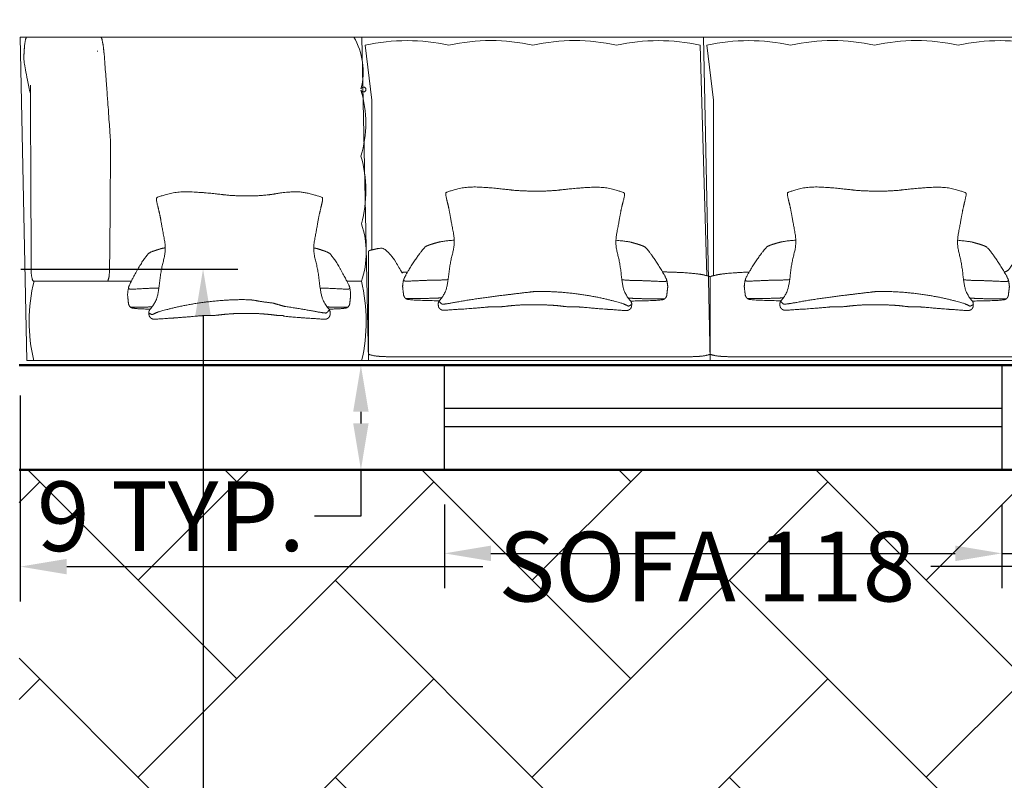
# Model space of a CAD drawing. Units: inches. Extents: x -466983 to 1020, y 324 to 318697.
# Tile 26 of 97: x 814 to 899, y 592 to 658. Entities that reach past the tile are written whole.
import ezdxf

# ---------------------------------------------------------------- set-up
doc = ezdxf.new("R2010")
doc.units = ezdxf.units.IN
doc.header["$MEASUREMENT"] = 0
for name, color, linetype, lineweight in [('A-ANNO-DIMS', 2, 'Continuous', 18), ('A-FLOR-PATT', 252, 'Continuous', 13), ('A-FURN', 8, 'Continuous', 18), ('A-GLAZ', 4, 'Continuous', 25), ('A-WALL', 7, 'Continuous', 50)]:
    doc.layers.add(name, color=color, linetype=linetype, lineweight=lineweight)
doc.styles.get("Standard").update_dxf_attribs({"font": 'arial.ttf'})
doc.dimstyles.get("Standard").update_dxf_attribs({"dimtxt": 6, "dimasz": 4, "dimexe": 3, "dimexo": 3, "dimgap": 0.09, "dimtad": 0, "dimtih": 1, "dimtoh": 1, "dimdec": 1, "dimzin": 0, "dimdsep": 46, "dimlunit": 3, "dimtxsty": 'Standard', "dimcen": 0.09, "dimadec": 0, "dimazin": 0, "dimtfac": 1, "dimtdec": 1, "dimtofl": 0, "dimtmove": 0, "dimatfit": 3, "dimfxl": 1, "dimtolj": 1, "dimtzin": 0, "dimarcsym": 0})

# ---------------------------------------------------------------- blocks, each defined once
blk = doc.blocks.new('Window 4 ft')
for p, q in [((1224.69, 893.769), (1233.69, 893.769)), ((1224.69, 845.769), (1224.69, 893.769)), ((1228.39, 845.769), (1228.39, 893.769)), ((1229.99, 893.769), (1229.99, 845.769)), ((1233.69, 893.769), (1233.69, 845.769)), ((1233.69, 845.769), (1224.69, 845.769))]:
    blk.add_line(p, q)
blk = doc.blocks.new('Sofa 1.1')
at = {"extrusion": (0, 0, -1)}
for p, q in [((2448.82, 970.73), (2401.83, 970.73)), ((2401.83, 970.73), (2402.74, 926.21)), ((2495.8, 970.73), (2448.82, 970.73)), ((2448.82, 970.73), (2449.73, 926.21)), ((2449.73, 926.21), (2448.82, 970.73)), ((2542.79, 970.73), (2495.8, 970.73)), ((2495.8, 970.73), (2496.71, 926.21)), ((2496.71, 926.21), (2495.8, 970.73)), ((2402.74, 926.21), (2449.73, 926.21)), ((2449.73, 926.21), (2496.71, 926.21)), ((2496.71, 926.21), (2543.7, 926.21))]:
    blk.add_line(p, q, dxfattribs=at)
for p, q in [((2448.82, 970.73), (2401.83, 970.73)), ((2401.83, 970.73), (2402.74, 926.21)), ((2495.8, 970.73), (2448.82, 970.73)), ((2448.82, 970.73), (2449.73, 926.21)), ((2449.73, 926.21), (2448.82, 970.73)), ((2449.27, 969.59), (2450.18, 962.03)), ((2496.26, 937.9), (2495.35, 969.59)), ((2542.79, 970.73), (2495.8, 970.73)), ((2495.8, 970.73), (2496.71, 926.21)), ((2496.71, 926.21), (2495.8, 970.73)), ((2496.26, 969.59), (2497.17, 962.03)), ((2450.18, 941.45), (2450.18, 962.03)), ((2497.17, 937.9), (2497.17, 962.03)), ((2413.76, 937.15), (2417.11, 937.15)), ((2446.75, 937.15), (2448.74, 937.15)), ((2402.74, 926.21), (2449.73, 926.21)), ((2449.73, 926.21), (2496.71, 926.21)), ((2496.71, 926.21), (2543.7, 926.21))]:
    blk.add_line(p, q)
for centre, radius, start, end in [((2439.61, 965.98), 9.38, 345.4157, 30.4474), ((2455.03, 943.99), 26.24, 77.3212, 102.6788), ((2466.55, 943.97), 26.27, 77.3353, 102.6728), ((2478.07, 943.97), 26.27, 77.3272, 102.6647), ((2489.59, 943.99), 26.24, 77.3212, 102.6788), ((2502.02, 943.99), 26.24, 77.3212, 102.6788), ((2513.54, 943.97), 26.27, 77.3353, 102.6728), ((2525.06, 943.97), 26.27, 77.3272, 102.6647), ((2536.58, 943.99), 26.24, 77.3212, 102.6788), ((2449.01, 963.51), 0.346, 198.7323, 161.2677), ((2433.87, 958.88), 15.49, 343.0329, 16.9671), ((2432.21, 949.59), 17.15, 344.5332, 16.1204), ((2437.6, 941.08), 11.82, 340.5487, 19.4513), ((2426.42, 931.59), 23.36, 166.2389, 193.3252), ((2426.05, 931.59), 23.36, 346.6748, 13.7611)]:
    blk.add_arc(centre, radius, start, end)
for points in [[(2402.42, 969.61), (2402.36, 968.74), (2402.33, 968.15), (2402.32, 967.24), (2403.22, 962.9)], [(2402.74, 970.73), (2402.57, 970.73), (2402.42, 969.61)], [(2412.89, 970.73), (2407.81, 970.73), (2402.74, 970.73)], [(2413.15, 969.97), (2413.03, 970.73), (2412.89, 970.73)], [(2413.33, 968.68), (2413.25, 969.67), (2413.15, 969.97)], [(2412.41, 968.79), (2412.43, 968.79), (2412.48, 968.78)], [(2413.37, 968.38), (2413.35, 968.53), (2413.33, 968.68)], [(2414.24, 956.06), (2414.28, 956.33), (2413.37, 968.38)], [(2403.22, 957.55), (2403.22, 953.33), (2403.22, 964.12)], [(2403.22, 964.12), (2403.23, 957.49), (2403.24, 956.59), (2403.27, 956), (2403.33, 938.27)], [(2403.22, 962.9), (2403.22, 961.77), (2403.22, 957.55)], [(2414.06, 937.91), (2414.16, 938.22), (2414.24, 956.06)], [(2430.1, 949), (2429.47, 949.07), (2427.17, 949.33), (2423.54, 949.52), (2420.73, 948.74), (2420.5, 948.54), (2420.73, 947.51), (2421.04, 946.25), (2421.35, 944.43), (2421.93, 941.46), (2421.17, 938.67), (2420.79, 935.09), (2420.13, 933.79), (2419.52, 933.11), (2419.51, 932.62), (2419.61, 932.2), (2420.08, 931.87), (2420.44, 931.91)], [(2443.53, 931.91), (2443.9, 931.87), (2444.36, 932.2), (2444.47, 932.62), (2444.45, 933.11), (2443.85, 933.79), (2443.18, 935.09), (2442.8, 938.67), (2442.04, 941.46), (2442.62, 944.43), (2442.93, 946.25), (2443.24, 947.51), (2443.47, 948.54), (2443.25, 948.74), (2440.43, 949.52), (2437.85, 949.33), (2436.39, 949.07), (2435.77, 949)], [(2460.21, 933.14), (2459.86, 933.11), (2459.41, 933.42), (2459.31, 933.83), (2459.32, 934.31), (2459.91, 934.96), (2460.56, 936.22), (2460.93, 939.68), (2461.67, 942.38), (2461.11, 945.25), (2460.81, 947.01), (2460.51, 948.24), (2460.29, 949.23), (2460.51, 949.43), (2463.24, 950.18), (2466.74, 949.98), (2468.97, 949.73), (2469.58, 949.66)], [(2475.7, 949.65), (2476.31, 949.72), (2478.54, 949.96), (2482.05, 950.15), (2484.77, 949.39), (2484.99, 949.19), (2484.77, 948.2), (2484.46, 946.98), (2484.16, 945.22), (2483.59, 942.34), (2484.32, 939.64), (2484.68, 936.18), (2485.33, 934.92), (2485.92, 934.26), (2485.93, 933.79), (2485.82, 933.38), (2485.37, 933.07), (2485.02, 933.1)], [(2507.2, 933.14), (2506.84, 933.11), (2506.4, 933.42), (2506.29, 933.83), (2506.31, 934.31), (2506.9, 934.96), (2507.54, 936.22), (2507.91, 939.68), (2508.65, 942.38), (2508.1, 945.25), (2507.8, 947.01), (2507.5, 948.24), (2507.28, 949.23), (2507.5, 949.43), (2510.22, 950.18), (2513.73, 949.98), (2515.96, 949.73), (2516.57, 949.66)], [(2522.69, 949.65), (2523.29, 949.72), (2525.53, 949.96), (2529.03, 950.15), (2531.76, 949.39), (2531.97, 949.19), (2531.75, 948.2), (2531.45, 946.98), (2531.14, 945.22), (2530.58, 942.34), (2531.31, 939.64), (2531.67, 936.18), (2532.32, 934.92), (2532.9, 934.26), (2532.91, 933.79), (2532.81, 933.38), (2532.36, 933.07), (2532.01, 933.1)], [(2450.45, 941.5), (2449.73, 941.38), (2449.73, 941.24)], [(2449.73, 941.24), (2449.73, 936.33), (2449.73, 927.16)], [(2403.33, 938.27), (2403.48, 937.15), (2403.65, 937.15)], [(2403.65, 937.15), (2408.72, 937.15), (2413.79, 937.15)], [(2413.79, 937.15), (2413.94, 937.15), (2414.06, 937.91)], [(2454.56, 937.34), (2454.56, 937.36), (2454.58, 937.41)], [(2490.73, 937.28), (2490.73, 937.31), (2490.72, 937.35)], [(2496.71, 937.7), (2496.71, 937.83), (2495.99, 937.96)], [(2497.44, 937.96), (2496.71, 937.83), (2496.71, 937.7)], [(2496.71, 937.7), (2496.71, 932.79), (2496.71, 927.16)], [(2496.71, 927.16), (2496.71, 932.79), (2496.71, 937.7)], [(2501.55, 937.34), (2501.55, 937.36), (2501.56, 937.41)], [(2416.72, 936.24), (2416.72, 936.26), (2416.73, 936.31)], [(2447.14, 936.24), (2447.14, 936.26), (2447.13, 936.31)], [(2433.96, 934.52), (2433.61, 934.57), (2433.26, 934.59)], [(2436.58, 934.13), (2435.05, 934.31), (2433.96, 934.52)], [(2459.42, 934.38), (2459.75, 934.01), (2459.86, 933.97)], [(2506.41, 934.38), (2506.73, 934.01), (2506.85, 933.97)], [(2438.19, 933.67), (2437.26, 933.94), (2436.58, 934.13)], [(2444.35, 933.18), (2444.01, 932.81), (2443.89, 932.76)], [(2468.93, 933.73), (2468.04, 933.6), (2466.54, 933.63), (2465.6, 933.53), (2462.58, 933.29), (2462.22, 933.29), (2460.21, 933.14)], [(2470.69, 933.87), (2469.72, 933.82), (2468.93, 933.73)], [(2476.3, 933.71), (2475.51, 933.81), (2474.54, 933.86)], [(2485.02, 933.1), (2483.01, 933.25), (2482.65, 933.26), (2479.63, 933.51), (2478.69, 933.61), (2477.2, 933.59), (2476.3, 933.71)], [(2485.48, 933.7), (2485.55, 933.73), (2485.92, 933.93)], [(2515.92, 933.73), (2515.02, 933.6), (2513.53, 933.63), (2512.59, 933.53), (2509.57, 933.29), (2509.21, 933.29), (2507.2, 933.14)], [(2517.68, 933.87), (2516.71, 933.82), (2515.92, 933.73)], [(2523.29, 933.71), (2522.5, 933.81), (2521.53, 933.86)], [(2532.01, 933.1), (2530, 933.25), (2529.63, 933.26), (2526.62, 933.51), (2525.68, 933.61), (2524.18, 933.59), (2523.29, 933.71)], [(2532.46, 933.7), (2532.54, 933.73), (2532.91, 933.93)], [(2419.97, 932.53), (2419.89, 932.56), (2419.51, 932.76)], [(2420.44, 931.91), (2422.52, 932.06), (2422.89, 932.07), (2426.01, 932.32), (2426.99, 932.42), (2428.53, 932.4), (2429.45, 932.53)], [(2429.45, 932.53), (2430.27, 932.62), (2431.27, 932.68)], [(2434.59, 932.68), (2435.59, 932.62), (2436.41, 932.53)], [(2436.41, 932.53), (2437.34, 932.4), (2438.03, 932.42), (2437.96, 932.32), (2441.08, 932.07), (2441.45, 932.06), (2443.53, 931.91)], [(2449.73, 927.16), (2449.73, 926.99), (2450.79, 926.85)], [(2450.79, 926.85), (2451.29, 926.79), (2451.86, 926.76), (2452.72, 926.75), (2459.03, 926.74)], [(2459.03, 926.74), (2468.57, 926.74), (2478.12, 926.74)], [(2478.12, 926.74), (2482.76, 926.74), (2487.41, 926.74)], [(2487.41, 926.74), (2493.72, 926.75), (2494.59, 926.76), (2495.15, 926.79), (2495.65, 926.85)], [(2495.65, 926.85), (2496.71, 926.99), (2496.71, 927.16)], [(2496.71, 927.16), (2496.71, 926.99), (2497.78, 926.85)], [(2497.78, 926.85), (2498.28, 926.79), (2498.84, 926.76), (2499.7, 926.75), (2506.02, 926.74)], [(2506.02, 926.74), (2515.56, 926.74), (2525.11, 926.74)], [(2525.11, 926.74), (2529.75, 926.74), (2534.4, 926.74)], [(2534.4, 926.74), (2540.71, 926.75), (2541.57, 926.76), (2542.13, 926.79), (2542.63, 926.85)]]:
    blk.add_open_spline(points, degree=2)
for points, knots in [([(2469.58, 949.66), (2470.85, 949.54), (2472.19, 949.54), (2472.42, 949.54), (2472.64, 949.54)], [50, 50, 50, 51, 51, 52, 52, 52]), ([(2472.64, 949.54), (2472.87, 949.54), (2473.09, 949.53), (2474.44, 949.53), (2475.7, 949.65)], [0, 0, 0, 1, 1, 2, 2, 2]), ([(2516.57, 949.66), (2517.83, 949.54), (2519.18, 949.54), (2519.4, 949.54), (2519.63, 949.54)], [50, 50, 50, 51, 51, 52, 52, 52]), ([(2519.63, 949.54), (2519.85, 949.54), (2520.08, 949.53), (2521.42, 949.53), (2522.69, 949.65)], [0, 0, 0, 1, 1, 2, 2, 2]), ([(2433.26, 948.87), (2433.03, 948.87), (2432.8, 948.87), (2431.41, 948.87), (2430.1, 949)], [0, 0, 0, 1, 1, 2, 2, 2]), ([(2435.77, 949), (2434.46, 948.87), (2433.73, 948.87), (2433.5, 948.87), (2433.26, 948.87)], [50, 50, 50, 51, 51, 52, 52, 52]), ([(2454.58, 937.41), (2454.66, 937.68), (2455.33, 938.79), (2456.12, 940.09), (2457.45, 941.86), (2457.92, 942.07), (2458.52, 942.28), (2459.45, 942.53), (2459.93, 942.65), (2461.51, 942.79)], [7, 7, 7, 8, 8, 9, 10, 11, 12, 12, 13, 13, 13]), ([(2483.76, 942.77), (2485.38, 942.62), (2485.87, 942.49), (2486.79, 942.23), (2487.39, 942.02), (2487.86, 941.81), (2489.19, 940.04), (2489.97, 938.74), (2490.64, 937.62), (2490.72, 937.35)], [0, 0, 0, 1, 1, 2, 3, 4, 5, 5, 6, 6, 6]), ([(2501.56, 937.41), (2501.64, 937.68), (2502.32, 938.79), (2503.1, 940.09), (2504.44, 941.86), (2504.91, 942.07), (2505.51, 942.28), (2506.43, 942.53), (2506.91, 942.65), (2508.49, 942.79)], [7, 7, 7, 8, 8, 9, 10, 11, 12, 12, 13, 13, 13]), ([(2530.74, 942.77), (2532.37, 942.62), (2532.85, 942.49), (2533.78, 942.23), (2534.38, 942.02), (2534.84, 941.81), (2536.18, 940.04), (2536.96, 938.74), (2537.63, 937.62), (2537.71, 937.35)], [0, 0, 0, 1, 1, 2, 3, 4, 5, 5, 6, 6, 6]), ([(2421.77, 941.73), (2421.36, 941.67), (2421.17, 941.61), (2420.32, 941.35), (2419.77, 941.13), (2419.35, 940.91), (2418.13, 939.08), (2417.42, 937.74), (2416.81, 936.59), (2416.73, 936.31)], [0, 0, 0, 1, 1, 2, 3, 4, 5, 5, 6, 6, 6]), ([(2447.13, 936.31), (2447.05, 936.59), (2446.44, 937.74), (2445.73, 939.08), (2444.51, 940.91), (2444.09, 941.13), (2443.54, 941.35), (2442.69, 941.61), (2442.52, 941.66), (2442.2, 941.71)], [6, 6, 6, 7, 7, 8, 9, 10, 11, 11, 12, 12, 12]), ([(2455.09, 938.39), (2454.69, 938.38), (2454.3, 938.36), (2452.43, 941.82), (2451.35, 941.68), (2450.74, 941.59), (2450.45, 941.5)], [0, 0, 0, 1, 1, 2, 2, 3, 3, 3]), ([(2542.98, 941.5), (2542.68, 941.59), (2542.08, 941.68), (2541, 941.82), (2539.13, 941.91), (2538.18, 938.4), (2537.14, 938.42)], [17, 17, 17, 18, 18, 19, 19, 20, 20, 20]), ([(2459.47, 934.45), (2459.36, 934.45), (2459.26, 934.45), (2456.53, 934.51), (2455.37, 934.6), (2454.89, 934.68), (2454.56, 935.07), (2454.5, 935.68), (2454.37, 936.65), (2454.58, 937.41)], [0, 0, 0, 1, 1, 2, 3, 4, 5, 6, 7, 7, 7]), ([(2454.56, 937.34), (2454.58, 937.18), (2454.97, 937.13), (2455.8, 937.18), (2458.16, 937.28), (2458.99, 937.28), (2459.7, 937.29), (2460.67, 937.36)], [0, 0, 0, 1, 2, 3, 4, 4, 5, 5, 5]), ([(2484.57, 937.33), (2485.57, 937.25), (2486.3, 937.24), (2487.13, 937.23), (2489.49, 937.13), (2490.32, 937.07), (2490.71, 937.13), (2490.73, 937.28)], [0, 0, 0, 1, 1, 2, 3, 4, 5, 5, 5]), ([(2490.72, 937.35), (2490.92, 936.59), (2490.79, 935.63), (2490.73, 935.01), (2490.4, 934.63), (2489.91, 934.55), (2488.75, 934.46), (2486.03, 934.41), (2485.9, 934.41), (2485.77, 934.41)], [6, 6, 6, 7, 8, 9, 10, 11, 12, 12, 13, 13, 13]), ([(2495.99, 937.96), (2495.7, 938.05), (2495.09, 938.13), (2494.01, 938.28), (2492.14, 938.36), (2491.19, 938.4), (2490.16, 938.42)], [17, 17, 17, 18, 18, 19, 19, 20, 20, 20]), ([(2502.08, 938.39), (2501.68, 938.38), (2501.28, 938.36), (2499.42, 938.28), (2498.34, 938.13), (2497.73, 938.05), (2497.44, 937.96)], [0, 0, 0, 1, 1, 2, 2, 3, 3, 3]), ([(2506.45, 934.45), (2506.35, 934.45), (2506.25, 934.45), (2503.52, 934.51), (2502.36, 934.6), (2501.88, 934.68), (2501.55, 935.07), (2501.49, 935.68), (2501.36, 936.65), (2501.56, 937.41)], [0, 0, 0, 1, 1, 2, 3, 4, 5, 6, 7, 7, 7]), ([(2501.55, 937.34), (2501.57, 937.18), (2501.96, 937.13), (2502.79, 937.18), (2505.15, 937.28), (2505.98, 937.28), (2506.69, 937.29), (2507.66, 937.36)], [0, 0, 0, 1, 2, 3, 4, 4, 5, 5, 5]), ([(2531.56, 937.33), (2532.56, 937.25), (2533.29, 937.24), (2534.12, 937.23), (2536.48, 937.13), (2537.31, 937.07), (2537.7, 937.13), (2537.72, 937.28)], [0, 0, 0, 1, 1, 2, 3, 4, 5, 5, 5]), ([(2537.71, 937.35), (2537.91, 936.59), (2537.77, 935.63), (2537.71, 935.01), (2537.39, 934.63), (2536.9, 934.55), (2535.74, 934.46), (2533.01, 934.41), (2532.88, 934.41), (2532.75, 934.41)], [6, 6, 6, 7, 8, 9, 10, 11, 12, 12, 13, 13, 13]), ([(2416.73, 936.31), (2416.55, 935.52), (2416.67, 934.53), (2416.72, 933.89), (2417.02, 933.49), (2417.47, 933.41), (2417.99, 933.36), (2418.36, 933.33), (2419.7, 933.29)], [6, 6, 6, 7, 8, 9, 10, 11, 11, 12, 12, 12]), ([(2420.9, 936.19), (2420.83, 936.19), (2420.76, 936.19), (2420, 936.18), (2417.85, 936.08), (2417.09, 936.02), (2416.74, 936.08), (2416.72, 936.24)], [0, 0, 0, 1, 1, 2, 3, 4, 5, 5, 5]), ([(2447.14, 936.24), (2447.12, 936.08), (2446.77, 936.02), (2446.01, 936.08), (2443.86, 936.18), (2443.1, 936.19), (2443.09, 936.19), (2443.07, 936.19)], [0, 0, 0, 1, 2, 3, 4, 4, 5, 5, 5]), ([(2444.27, 933.3), (2445.51, 933.33), (2445.87, 933.36), (2446.4, 933.41), (2446.84, 933.49), (2447.14, 933.89), (2447.19, 934.53), (2447.31, 935.52), (2447.13, 936.31)], [0, 0, 0, 1, 1, 2, 3, 4, 5, 6, 6, 6]), ([(2472.62, 935.72), (2475.03, 935.78), (2477.67, 935.48), (2480.31, 935.17), (2482.38, 934.68), (2484.45, 934.18), (2484.87, 933.99), (2485.27, 933.81), (2485.41, 933.73), (2485.45, 933.71), (2485.48, 933.7)], [6, 6, 6, 7, 7, 8, 8, 9, 9, 10, 10, 11, 11, 11]), ([(2519.61, 935.72), (2522.01, 935.78), (2524.66, 935.48), (2527.3, 935.17), (2529.36, 934.68), (2531.44, 934.18), (2531.85, 933.99), (2532.26, 933.81), (2532.39, 933.73), (2532.43, 933.71), (2532.46, 933.7)], [6, 6, 6, 7, 7, 8, 8, 9, 9, 10, 10, 11, 11, 11]), ([(2433.26, 934.59), (2430.77, 934.66), (2428.04, 934.35), (2425.31, 934.04), (2423.18, 933.53), (2421.03, 933.02), (2420.6, 932.83), (2420.18, 932.64), (2420.04, 932.56), (2420, 932.54), (2419.97, 932.53)], [6, 6, 6, 7, 7, 8, 8, 9, 9, 10, 10, 11, 11, 11]), ([(2459.79, 934.85), (2459.05, 934.81), (2458.37, 934.79), (2457.06, 934.76), (2456.34, 934.76), (2455.77, 934.76), (2454.83, 934.77)], [0, 0, 0, 1, 1, 2, 2, 3, 3, 3]), ([(2459.86, 933.97), (2460.15, 933.96), (2461.71, 934.24), (2463.48, 934.57), (2465.38, 934.83), (2467.28, 935.1), (2468.77, 935.27), (2470.25, 935.45), (2471.94, 935.65), (2472.28, 935.69), (2472.62, 935.72)], [1, 1, 1, 2, 2, 3, 3, 4, 4, 5, 5, 6, 6, 6]), ([(2490.46, 934.72), (2489.52, 934.71), (2488.95, 934.71), (2488.23, 934.71), (2486.92, 934.75), (2486.21, 934.77), (2485.44, 934.82)], [0, 0, 0, 1, 1, 2, 2, 3, 3, 3]), ([(2506.78, 934.85), (2506.04, 934.81), (2505.36, 934.79), (2504.04, 934.76), (2503.33, 934.76), (2502.75, 934.76), (2501.82, 934.77)], [0, 0, 0, 1, 1, 2, 2, 3, 3, 3]), ([(2506.85, 933.97), (2507.13, 933.96), (2508.69, 934.24), (2510.47, 934.57), (2512.37, 934.83), (2514.27, 935.1), (2515.76, 935.27), (2517.24, 935.45), (2518.93, 935.65), (2519.27, 935.69), (2519.61, 935.72)], [1, 1, 1, 2, 2, 3, 3, 4, 4, 5, 5, 6, 6, 6]), ([(2537.44, 934.72), (2536.51, 934.71), (2535.94, 934.71), (2535.22, 934.71), (2533.9, 934.75), (2533.2, 934.77), (2532.43, 934.82)], [0, 0, 0, 1, 1, 2, 2, 3, 3, 3]), ([(2416.97, 933.59), (2417.82, 933.57), (2418.35, 933.57), (2418.93, 933.57), (2419.95, 933.61)], [0, 0, 0, 1, 1, 2, 2, 2]), ([(2443.89, 932.76), (2443.6, 932.75), (2441.99, 933.05), (2440.16, 933.39), (2438.19, 933.67)], [1, 1, 1, 2, 2, 3, 3, 3]), ([(2444.02, 933.6), (2444.96, 933.57), (2445.51, 933.57), (2446.04, 933.57), (2446.89, 933.59)], [0, 0, 0, 1, 1, 2, 2, 2]), ([(2474.54, 933.86), (2473.81, 933.88), (2473.06, 933.88), (2472.62, 933.88), (2472.18, 933.88), (2471.43, 933.88), (2470.69, 933.87)], [24, 24, 24, 25, 25, 27, 27, 28, 28, 28]), ([(2521.53, 933.86), (2520.79, 933.88), (2520.04, 933.88), (2519.6, 933.88), (2519.16, 933.88), (2518.41, 933.88), (2517.68, 933.87)], [24, 24, 24, 25, 25, 27, 27, 28, 28, 28]), ([(2431.27, 932.68), (2432.03, 932.69), (2432.81, 932.69), (2433.26, 932.69), (2433.72, 932.69), (2434.49, 932.69), (2434.59, 932.68)], [24, 24, 24, 25, 25, 27, 27, 28, 28, 28])]:
    blk.add_open_spline(points, degree=2, knots=knots)
blk = doc.blocks.new('*D59')
at = {"layer": 'A-ANNO-DIMS', "color": 0, "lineweight": -2, "transparency": 16777216}
for p, q in [((850.445, 615.938), (850.445, 608.738)), ((898.445, 615.938), (898.445, 608.738)), ((854.445, 611.738), (894.445, 611.738)), ((898.445, 611.738), (902.445, 611.738))]:
    blk.add_line(p, q, dxfattribs=at)
at = {"layer": 'A-ANNO-DIMS', "color": 0, "transparency": 16777216}
for points in [[(854.445, 612.404), (854.445, 611.071), (850.445, 611.738)], [(894.445, 612.404), (894.445, 611.071), (898.445, 611.738)]]:
    blk.add_solid(points, dxfattribs=at)
at = {"layer": 'Defpoints', "color": 0, "transparency": 16777216}
for p in [(850.445, 618.938), (898.445, 618.938), (898.445, 611.738)]:
    blk.add_point(p, dxfattribs=at)
at = {"layer": 'A-ANNO-DIMS', "color": 0, "transparency": 16777216, "insert": (941.109, 611.738), "char_height": 6, "attachment_point": 5}
blk.add_mtext("\\A1;WINDOW 4' 48 TYP.", dxfattribs=at)
blk = doc.blocks.new('*D60')
at = {"layer": 'A-ANNO-DIMS', "color": 0, "lineweight": -2, "transparency": 16777216}
for p, q in [((847.445, 627.938), (840.245, 627.938)), ((843.245, 623.938), (843.245, 622.938)), ((847.445, 618.938), (840.245, 618.938)), ((843.245, 618.938), (843.245, 614.938)), ((843.245, 614.938), (839.245, 614.938))]:
    blk.add_line(p, q, dxfattribs=at)
at = {"layer": 'A-ANNO-DIMS', "color": 0, "transparency": 16777216}
for points in [[(842.578, 623.938), (843.911, 623.938), (843.245, 627.938)], [(842.578, 622.938), (843.911, 622.938), (843.245, 618.938)]]:
    blk.add_solid(points, dxfattribs=at)
at = {"layer": 'Defpoints', "color": 0, "transparency": 16777216}
for p in [(850.445, 627.938), (843.245, 618.938), (850.445, 618.938)]:
    blk.add_point(p, dxfattribs=at)
at = {"layer": 'A-ANNO-DIMS', "color": 0, "transparency": 16777216, "insert": (826.883, 614.938), "char_height": 6, "attachment_point": 5}
blk.add_mtext('\\A1;9 TYP.', dxfattribs=at)
blk = doc.blocks.new('*D69')
at = {"layer": 'A-ANNO-DIMS', "color": 0, "lineweight": -2, "transparency": 16777216}
for p, q in [((813.968, 636.229), (832.65, 636.229)), ((829.65, 632.229), (829.65, 577.152)), ((829.65, 515.686), (829.65, 570.763)), ((813.968, 511.686), (832.65, 511.686))]:
    blk.add_line(p, q, dxfattribs=at)
at = {"layer": 'A-ANNO-DIMS', "color": 0, "transparency": 16777216}
for points in [[(828.983, 632.229), (830.316, 632.229), (829.65, 636.229)], [(828.983, 515.686), (830.316, 515.686), (829.65, 511.686)]]:
    blk.add_solid(points, dxfattribs=at)
at = {"layer": 'Defpoints', "color": 0, "transparency": 16777216}
for p in [(810.968, 636.229), (829.65, 636.229), (810.968, 511.686)]:
    blk.add_point(p, dxfattribs=at)
at = {"layer": 'A-ANNO-DIMS', "color": 0, "transparency": 16777216, "insert": (829.65, 573.958), "char_height": 6, "attachment_point": 5}
blk.add_mtext('\\A1;L-SOFA 125', dxfattribs=at)
blk = doc.blocks.new('*D103')
at = {"layer": 'A-ANNO-DIMS', "color": 0, "lineweight": -2, "transparency": 16777216}
for p, q in [((813.905, 625.338), (813.905, 607.596)), ((932.185, 625.338), (932.185, 607.596)), ((817.905, 610.596), (853.76, 610.596)), ((928.185, 610.596), (892.33, 610.596))]:
    blk.add_line(p, q, dxfattribs=at)
at = {"layer": 'A-ANNO-DIMS', "color": 0, "transparency": 16777216}
for points in [[(817.905, 611.262), (817.905, 609.929), (813.905, 610.596)], [(928.185, 611.262), (928.185, 609.929), (932.185, 610.596)]]:
    blk.add_solid(points, dxfattribs=at)
at = {"layer": 'Defpoints', "color": 0, "transparency": 16777216}
for p in [(813.905, 628.338), (932.185, 628.338), (932.185, 610.596)]:
    blk.add_point(p, dxfattribs=at)
at = {"layer": 'A-ANNO-DIMS', "color": 0, "transparency": 16777216, "insert": (873.045, 610.596), "char_height": 6, "attachment_point": 5}
blk.add_mtext('\\A1;SOFA 118', dxfattribs=at)

msp = doc.modelspace()

# ---------------------------------------------------------------- hatches: boundary and pattern name
at = {"layer": 'A-FLOR-PATT', "transparency": 33554572}
h = msp.add_hatch(dxfattribs=at)
h.set_pattern_fill('ANSI37', color=256, scale=30)
h.set_pattern_definition([(45, (-1212.4137, -290.035), (-2.6516504, 2.6516504), []), (135, (-1212.4137, -290.035), (-2.6516504, -2.6516504), [])])
h.paths.add_polyline_path([(901.806, 1075.938), (900.614, 1075.938), (900.614, 1065.386), (899.391, 1065.386), (898.091, 1065.386), (892.836, 1058.71, -0.258377), (892.188, 1058.351), (879.985, 1058.351, -0.20177), (879.438, 1058.581), (874.081, 1065.386), (872.781, 1065.386), (871.558, 1065.386), (871.558, 1075.938), (813.806, 1075.938), (813.806, 1044.792), (832.395, 1044.792, -0.394795), (848.66, 1028.536), (848.66, 1009.938), (901.806, 1009.938), (901.806, 1015.938), (901.306, 1015.938), (871.306, 1015.938), (871.306, 1017.25), (871.334, 1017.25, -0.401453), (901.306, 1045.938), (901.806, 1045.938)])
edge = h.paths.add_edge_path(flags=16)
edge.add_line((847.773, 1068.949), (847.773, 1073.709))
edge.add_arc((849.227, 1073.709), 1.454, 90, 180, ccw=False)
edge.add_line((849.227, 1075.163), (864.492, 1075.163))
edge.add_arc((864.492, 1073.709), 1.454, 0, 90, ccw=False)
edge.add_line((865.946, 1073.709), (865.946, 1069.004))
edge.add_arc((832.645, 1068.976), 33.301, -20.61234, 0.04725, ccw=False)
edge.add_ellipse((856.859, 1058.48), major_axis=(0, 10.213), ratio=0.685919, start_angle=100.00884, end_angle=259.99116, ccw=False)
edge.add_arc((881.074, 1068.976), 33.301, 180.04725, 200.61234, ccw=False)
h.paths.add_polyline_path([(853.146, 1066.482), (853.146, 1066.453), (853.146, 1066.453, 0.433107), (852.917, 1066.685), (852.917, 1066.453), (853.146, 1066.453), (853.146, 1066.482), (853.088, 1066.612, 0.697939), (852.7, 1066.453), (852.7, 1066.453), (852.7, 1066.482), (852.917, 1067.001), (852.917, 1066.685, -0.396254)], flags=0)
h.paths.add_polyline_path([(861.019, 1066.482), (861.019, 1066.453), (861.019, 1066.453, 0.416404), (860.802, 1066.685), (860.802, 1066.453), (861.019, 1066.453), (861.019, 1066.482), (860.967, 1066.605, 0.713344), (860.573, 1066.453), (860.573, 1066.453), (860.573, 1066.482), (860.802, 1067.001), (860.802, 1066.685, -0.379973)], flags=0)
edge = h.paths.add_edge_path(flags=0)
edge.add_spline(control_points=[(861.13, 1065.785), (861.466, 1065.248), (861.613, 1065.016), (861.983, 1064.374), (862.192, 1063.944), (862.561, 1063.039), (862.721, 1062.563), (862.987, 1061.578), (863.092, 1061.069), (863.245, 1060.031), (863.293, 1059.503), (863.329, 1058.441), (863.318, 1057.908), (863.237, 1056.852), (863.166, 1056.329), (862.97, 1055.308), (862.843, 1054.81), (862.537, 1053.852), (862.357, 1053.393), (861.951, 1052.525), (861.725, 1052.117), (861.233, 1051.362), (860.967, 1051.016), (860.405, 1050.395), (860.108, 1050.12), (859.494, 1049.646), (859.176, 1049.448), (858.528, 1049.13), (858.197, 1049.011), (857.531, 1048.852), (857.196, 1048.812), (856.525, 1048.812), (856.189, 1048.852), (855.524, 1049.01), (855.193, 1049.129), (854.545, 1049.447), (854.227, 1049.645), (853.612, 1050.118), (853.316, 1050.393), (852.753, 1051.014), (852.487, 1051.36), (851.995, 1052.114), (851.769, 1052.523), (851.363, 1053.39), (851.183, 1053.85), (850.877, 1054.807), (850.75, 1055.305), (850.553, 1056.326), (850.483, 1056.849), (850.401, 1057.905), (850.39, 1058.438), (850.426, 1059.5), (850.473, 1060.028), (850.626, 1061.066), (850.732, 1061.575), (850.997, 1062.561), (851.157, 1063.036), (851.525, 1063.942), (851.734, 1064.371), (852.106, 1065.016), (852.254, 1065.25), (852.608, 1065.733)], knot_values=[3.915332, 3.915332, 3.915332, 3.915332, 4.013468, 4.013468, 4.175532, 4.175532, 4.337596, 4.337596, 4.49966, 4.49966, 4.661724, 4.661724, 4.823788, 4.823788, 4.985852, 4.985852, 5.147916, 5.147916, 5.30998, 5.30998, 5.472044, 5.472044, 5.634109, 5.634109, 5.796173, 5.796173, 5.958237, 5.958237, 6.120301, 6.120301, 6.282365, 6.282365, 6.444429, 6.444429, 6.606493, 6.606493, 6.768557, 6.768557, 6.930621, 6.930621, 7.092685, 7.092685, 7.254749, 7.254749, 7.416813, 7.416813, 7.578878, 7.578878, 7.740942, 7.740942, 7.903006, 7.903006, 8.06507, 8.06507, 8.227134, 8.227134, 8.389198, 8.389198, 8.551262, 8.551262, 8.65037, 8.65037, 8.65037, 8.65037], degree=3, periodic=0)
edge.add_line((852.642, 1065.785), (861.13, 1065.785))
edge = h.paths.add_edge_path(flags=0)
edge.add_ellipse((856.85, 1057.743), major_axis=(0, 7.792), ratio=0.687861, start_angle=0, end_angle=360)
h.paths.add_polyline_path([(848.863, 1069.389), (848.863, 1073.96, -0.414214), (849.954, 1075.051), (863.765, 1075.051, -0.414214), (864.856, 1073.96), (864.856, 1069.389, -0.388936), (864.524, 1069.027, -0.043561), (849.195, 1069.027, -0.388936)], flags=0)
h.paths.add_polyline_path([(853.101, 1068.112, -1), (852.677, 1068.112, -1)], flags=0)
edge = h.paths.add_edge_path(flags=0)
edge.add_ellipse((856.859, 1057.338), major_axis=(0, 2.207), ratio=0.657164, start_angle=0, end_angle=360)
h.paths.add_polyline_path([(861.041, 1068.112, -1), (860.618, 1068.112, -1)], flags=0)
edge = h.paths.add_edge_path()
edge.add_line((573.954, 1057.341), (573.954, 1075.938))
edge.add_line((573.954, 1075.938), (558.731, 1075.938))
edge.add_line((558.731, 1075.938), (558.731, 1065.386))
edge.add_line((558.731, 1065.386), (557.507, 1065.386))
edge.add_line((557.507, 1065.386), (556.207, 1065.386))
edge.add_line((556.207, 1065.386), (550.952, 1058.71))
edge.add_arc((550.304, 1059.116), 0.765, 270, 327.94832, ccw=False)
edge.add_line((550.304, 1058.351), (538.101, 1058.351))
edge.add_arc((538.101, 1059.116), 0.765, 224.3704, 270, ccw=False)
edge.add_line((537.555, 1058.581), (532.198, 1065.386))
edge.add_line((532.198, 1065.386), (530.898, 1065.386))
edge.add_line((530.898, 1065.386), (529.674, 1065.386))
edge.add_line((529.674, 1065.386), (529.674, 1075.938))
edge.add_line((529.674, 1075.938), (520.806, 1075.938))
edge.add_line((520.806, 1075.938), (520.806, 1045.938))
edge.add_line((520.806, 1045.938), (521.306, 1045.938))
edge.add_arc((521.306, 1015.938), 30, 2.50749, 90, ccw=False)
edge.add_line((551.277, 1017.25), (551.306, 1017.25))
edge.add_line((551.306, 1017.25), (551.306, 1015.938))
edge.add_line((551.306, 1015.938), (520.806, 1015.938))
edge.add_line((520.806, 1015.938), (520.806, 1009.938))
edge.add_line((520.806, 1009.938), (559.191, 1010.402))
edge.add_arc((559.191, 1011.856), 1.454, 180, 270, ccw=False)
edge.add_line((557.737, 1011.856), (557.737, 1016.561))
edge.add_arc((591.039, 1016.589), 33.301, 159.38766, 180.04725, ccw=False)
edge.add_ellipse((566.824, 1027.085), major_axis=(0, 10.213), ratio=0.685919, start_angle=280.00884, end_angle=439.99116, ccw=False)
edge.add_arc((542.609, 1016.589), 33.301, 0.04725, 20.61234, ccw=False)
edge.add_line((575.91, 1016.616), (575.91, 1011.856))
edge.add_arc((574.456, 1011.856), 1.454, -90, 0, ccw=False)
edge.add_line((574.456, 1010.402), (608.806, 1009.938))
edge.add_line((608.806, 1009.938), (608.806, 1041.086))
edge.add_line((608.806, 1041.086), (590.218, 1041.086))
edge.add_arc((590.775, 1057.907), 16.831, 181.92775, 268.10321, ccw=False)
edge = h.paths.add_edge_path()
edge.add_ellipse((494.244, 583.62), major_axis=(0, 10.213), ratio=0.685919, start_angle=280.00884, end_angle=439.99116, ccw=False)
edge.add_arc((470.03, 573.124), 33.301, 0.04725, 20.61234, ccw=False)
edge.add_line((503.331, 573.152), (503.331, 568.392))
edge.add_arc((501.877, 568.392), 1.454, -90, 0, ccw=False)
edge.add_line((501.877, 566.938), (539.806, 566.938))
edge.add_line((539.806, 566.938), (539.806, 572.938))
edge.add_line((539.806, 572.938), (539.306, 572.938))
edge.add_line((539.306, 572.938), (509.306, 572.938))
edge.add_line((509.306, 572.938), (509.306, 574.25))
edge.add_line((509.306, 574.25), (509.334, 574.25))
edge.add_arc((539.306, 572.938), 30, 90, 177.49251, ccw=False)
edge.add_line((539.306, 602.938), (539.806, 602.938))
edge.add_line((539.806, 602.938), (539.806, 626.938))
edge.add_line((539.806, 626.938), (531.772, 626.938))
edge.add_line((531.772, 626.938), (531.772, 616.386))
edge.add_line((531.772, 616.386), (530.548, 616.386))
edge.add_line((530.548, 616.386), (529.249, 616.386))
edge.add_line((529.249, 616.386), (523.711, 609.351))
edge.add_line((523.711, 609.351), (510.777, 609.351))
edge.add_line((510.777, 609.351), (505.239, 616.386))
edge.add_line((505.239, 616.386), (503.939, 616.386))
edge.add_line((503.939, 616.386), (502.715, 616.386))
edge.add_line((502.715, 616.386), (502.715, 626.938))
edge.add_line((502.715, 626.938), (481.698, 626.938))
edge.add_line((481.698, 626.938), (481.698, 610.995))
edge.add_arc((467.27, 611.473), 14.436, 271.92775, 358.10321, ccw=False)
edge.add_line((467.756, 597.045), (451.806, 597.045))
edge.add_line((451.806, 597.045), (451.806, 584.404))
edge.add_line((451.806, 584.404), (451.806, 566.938))
edge.add_line((451.806, 566.938), (486.612, 566.938))
edge.add_arc((486.612, 568.392), 1.454, 180, 270, ccw=False)
edge.add_line((485.158, 568.392), (485.158, 573.097))
edge.add_arc((518.459, 573.124), 33.301, 159.38766, 180.04725, ccw=False)
h.paths.add_polyline_path([(836.261, 1020.733), (879.89, 1020.733), (879.89, 1039.39), (836.261, 1039.39)], flags=25)
h.paths.add_polyline_path([(549.985, 1036.749), (593.614, 1036.749), (593.614, 1055.407), (549.985, 1055.407)], flags=24)
h.paths.add_polyline_path([(475.123, 595.596), (518.752, 595.596), (518.752, 614.253), (475.123, 614.253)], flags=24)
h = msp.add_hatch(dxfattribs=at)
h.set_pattern_fill('AR-HBONE', color=256, scale=3)
h.set_pattern_definition([(45, (-1212.414, -290.035), (0, 16.97056), [36, -12]), (135, (-1203.928, -281.55), (1e-15, 16.97056), [36, -12])])
h.paths.add_polyline_path([(987.806, 618.938), (813.806, 618.938), (813.806, 368.938), (987.806, 368.938)])

# ---------------------------------------------------------------- linework, layer by layer
at = {"layer": 'A-WALL'}
for p, q in [((934.806, 627.938), (813.806, 627.938)), ((934.806, 618.938), (813.806, 618.938))]:
    msp.add_line(p, q, dxfattribs=at)

# ---------------------------------------------------------------- block references
at = {"layer": 'A-FURN', "xscale": 0.6262868215902297, "yscale": 0.6262868215902297, "zscale": 0.6262868215902297}
msp.add_blockref('Sofa 1.1', (-690.329, 48.267), dxfattribs=at)
at = {"layer": 'A-GLAZ', "rotation": 270}
msp.add_blockref('Window 4 ft', (4.676, 1852.628), dxfattribs=at)

# ---------------------------------------------------------------- dimensions: what is measured, and where the dimension line sits
at = {"layer": 'A-ANNO-DIMS'}
for base, p1, p2, angle, text, picture, middle in [((829.65, 636.229), (810.968, 511.686), (810.968, 636.229), 90, 'L-SOFA <>', '*D69', (829.65, 573.958)), ((843.245, 618.938), (850.445, 627.938), (850.445, 618.938), 270, '<> TYP.', '*D60', (826.883, 614.938))]:
    dim = msp.add_linear_dim(base=base, p1=p1, p2=p2, angle=angle, text=text, dimstyle='Standard', override={"dimdec": 0, "dimlfac": 1, "dimrnd": 0, "dimzin": 0, "dimdsep": 46, "dimlunit": 2}, dxfattribs=at)
    dim.commit()
    dim.dimension.update_dxf_attribs({"geometry": picture, "text_midpoint": middle})
for base, p1, p2, text, picture, middle in [((898.445, 611.738), (850.445, 618.938), (898.445, 618.938), "WINDOW 4' <> TYP.", '*D59', (941.109, 611.738)), ((932.185, 610.596), (813.905, 628.338), (932.185, 628.338), 'SOFA <>', '*D103', (873.045, 610.596))]:
    dim = msp.add_linear_dim(base=base, p1=p1, p2=p2, text=text, dimstyle='Standard', override={"dimdec": 0, "dimlfac": 1, "dimrnd": 0, "dimzin": 0, "dimdsep": 46, "dimlunit": 2}, dxfattribs=at)
    dim.commit()
    dim.dimension.update_dxf_attribs({"geometry": picture, "text_midpoint": middle})

doc.saveas('drawing.dxf')
